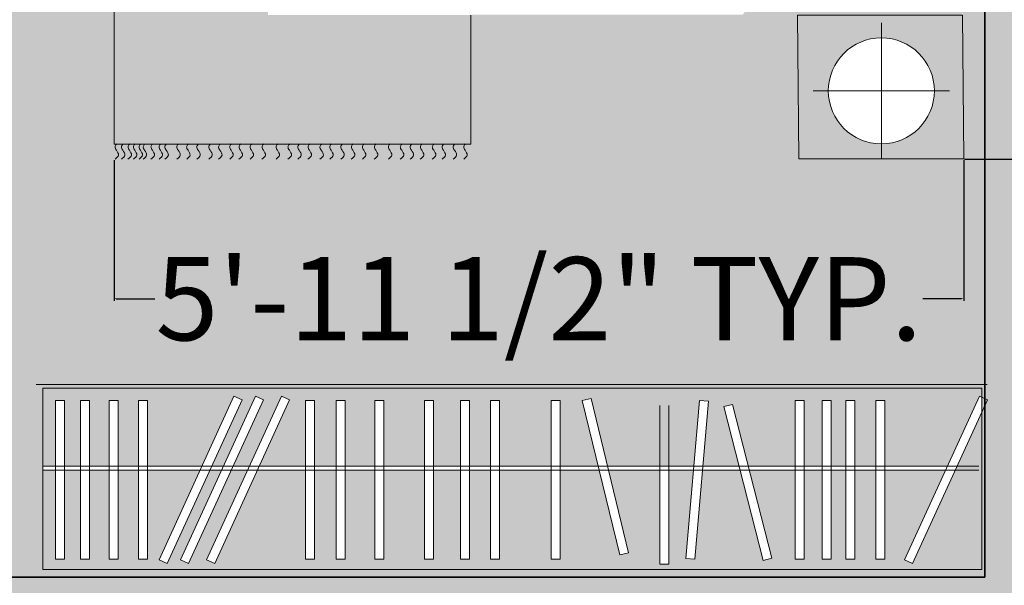
# Model space of a CAD drawing. Units: inches. Extents: x 1316 to 1777, y 813 to 1650.
# Tile 19 of 22: x 1623 to 1706, y 1434 to 1481. Entities that reach past the tile are written whole.
import ezdxf

# ---------------------------------------------------------------- set-up
doc = ezdxf.new("R2010")
doc.units = ezdxf.units.IN
doc.header["$MEASUREMENT"] = 0
for name, color, linetype, lineweight in [('A-ANNO-DIMS', 2, 'Continuous', 18), ('A-FLOR-CASE-PATT', 252, 'Continuous', 13), ('A-FURN-PATT', 23, 'Continuous', 13), ('A-WALL-PATT', 250, 'Continuous', 13), ('closet', 23, 'Continuous', 18), ('furniture', 23, 'Continuous', 18), ('walls', 250, 'Continuous', 35)]:
    doc.layers.add(name, color=color, linetype=linetype, lineweight=lineweight)
doc.layers.add('A-FLOR-PATT', color=254, linetype='Continuous', lineweight=13, true_color=0xfeeab9)
doc.styles.get("Standard").update_dxf_attribs({"font": 'arial.ttf'})
doc.dimstyles.get("Standard").update_dxf_attribs({"dimtxt": 7, "dimasz": 0.18, "dimexe": 0.18, "dimexo": 0.0625, "dimgap": 0.09, "dimtad": 0, "dimtih": 1, "dimtoh": 1, "dimzin": 0, "dimdsep": 46, "dimlunit": 3, "dimtxsty": 'Standard', "dimcen": 0.09, "dimadec": 0, "dimazin": 0, "dimtfac": 1, "dimtofl": 0, "dimtmove": 0, "dimatfit": 3, "dimfxl": 1, "dimtolj": 1, "dimtzin": 0, "dimarcsym": 0})

# ---------------------------------------------------------------- blocks, each defined once
blk = doc.blocks.new('CARPET')
at = {"layer": 'furniture'}
for p, q in [((36, -55.12), (51.55, -55.12)), ((51.55, -55.12), (51.55, -98.11)), ((51.55, -98.11), (-51.53, -98.11))]:
    blk.add_line(p, q, dxfattribs=at)
for points, knots in [([(53.37, -55.99), (53.22, -55.8), (52.9, -55.41), (52.34, -55.8), (51.89, -56.08), (51.65, -55.91), (51.53, -55.83)], [0, 0, 0, 0, 0.653278, 1.290138, 1.740457, 2.114451, 2.114451, 2.114451, 2.114451]), ([(53.37, -57.26), (53.22, -57.07), (52.9, -56.67), (52.34, -57.07), (51.89, -57.35), (51.65, -57.17), (51.53, -57.1)], [0, 0, 0, 0, 0.653278, 1.290138, 1.740457, 2.114451, 2.114451, 2.114451, 2.114451]), ([(53.37, -58.59), (53.22, -58.4), (52.9, -58.01), (52.34, -58.4), (51.89, -58.68), (51.65, -58.5), (51.53, -58.43)], [0, 0, 0, 0, 0.653278, 1.290138, 1.740457, 2.114451, 2.114451, 2.114451, 2.114451]), ([(53.37, -59.78), (53.22, -59.58), (52.9, -59.19), (52.34, -59.58), (51.89, -59.86), (51.65, -59.69), (51.53, -59.61)], [0, 0, 0, 0, 0.653278, 1.290138, 1.740457, 2.114451, 2.114451, 2.114451, 2.114451]), ([(53.37, -61.22), (53.22, -61.02), (52.9, -60.63), (52.34, -61.02), (51.89, -61.3), (51.65, -61.13), (51.53, -61.05)], [0, 0, 0, 0, 0.653278, 1.290138, 1.740457, 2.114451, 2.114451, 2.114451, 2.114451]), ([(53.37, -62.44), (53.22, -62.25), (52.9, -61.86), (52.34, -62.25), (51.89, -62.53), (51.65, -62.36), (51.53, -62.28)], [0, 0, 0, 0, 0.653278, 1.290138, 1.740457, 2.114451, 2.114451, 2.114451, 2.114451]), ([(53.37, -63.63), (53.22, -63.43), (52.9, -63.04), (52.34, -63.43), (51.89, -63.72), (51.65, -63.54), (51.53, -63.46)], [0, 0, 0, 0, 0.653278, 1.290138, 1.740457, 2.114451, 2.114451, 2.114451, 2.114451]), ([(53.37, -65.07), (53.22, -64.87), (52.9, -64.48), (52.34, -64.87), (51.89, -65.15), (51.65, -64.98), (51.53, -64.9)], [0, 0, 0, 0, 0.653278, 1.290138, 1.740457, 2.114451, 2.114451, 2.114451, 2.114451]), ([(53.37, -66.76), (53.22, -66.56), (52.9, -66.17), (52.34, -66.56), (51.89, -66.84), (51.65, -66.67), (51.53, -66.59)], [0, 0, 0, 0, 0.653278, 1.290138, 1.740457, 2.114451, 2.114451, 2.114451, 2.114451]), ([(53.37, -68.2), (53.22, -68), (52.9, -67.61), (52.34, -68), (51.89, -68.28), (51.65, -68.11), (51.53, -68.03)], [0, 0, 0, 0, 0.653278, 1.290138, 1.740457, 2.114451, 2.114451, 2.114451, 2.114451]), ([(53.37, -69.53), (53.22, -69.33), (52.9, -68.94), (52.34, -69.33), (51.89, -69.61), (51.65, -69.44), (51.53, -69.36)], [0, 0, 0, 0, 0.653278, 1.290138, 1.740457, 2.114451, 2.114451, 2.114451, 2.114451]), ([(53.37, -70.79), (53.22, -70.6), (52.9, -70.21), (52.34, -70.6), (51.89, -70.88), (51.65, -70.7), (51.53, -70.63)], [0, 0, 0, 0, 0.653278, 1.290138, 1.740457, 2.114451, 2.114451, 2.114451, 2.114451]), ([(53.37, -72.12), (53.22, -71.93), (52.9, -71.54), (52.34, -71.93), (51.89, -72.21), (51.65, -72.04), (51.53, -71.96)], [0, 0, 0, 0, 0.653278, 1.290138, 1.740457, 2.114451, 2.114451, 2.114451, 2.114451]), ([(53.37, -73.31), (53.22, -73.11), (52.9, -72.72), (52.34, -73.11), (51.89, -73.4), (51.65, -73.22), (51.53, -73.14)], [0, 0, 0, 0, 0.653278, 1.290138, 1.740457, 2.114451, 2.114451, 2.114451, 2.114451]), ([(53.37, -74.75), (53.22, -74.55), (52.9, -74.16), (52.34, -74.55), (51.89, -74.83), (51.65, -74.66), (51.53, -74.58)], [0, 0, 0, 0, 0.653278, 1.290138, 1.740457, 2.114451, 2.114451, 2.114451, 2.114451]), ([(53.37, -75.98), (53.22, -75.78), (52.9, -75.39), (52.34, -75.78), (51.89, -76.06), (51.65, -75.89), (51.53, -75.81)], [0, 0, 0, 0, 0.653278, 1.290138, 1.740457, 2.114451, 2.114451, 2.114451, 2.114451]), ([(53.37, -77.16), (53.22, -76.96), (52.9, -76.57), (52.34, -76.96), (51.89, -77.25), (51.65, -77.07), (51.53, -76.99)], [0, 0, 0, 0, 0.653278, 1.290138, 1.740457, 2.114451, 2.114451, 2.114451, 2.114451]), ([(53.37, -78.6), (53.22, -78.4), (52.9, -78.01), (52.34, -78.4), (51.89, -78.68), (51.65, -78.51), (51.53, -78.43)], [0, 0, 0, 0, 0.653278, 1.290138, 1.740457, 2.114451, 2.114451, 2.114451, 2.114451]), ([(53.37, -80.29), (53.22, -80.09), (52.9, -79.7), (52.34, -80.09), (51.89, -80.37), (51.65, -80.2), (51.53, -80.12)], [0, 0, 0, 0, 0.653278, 1.290138, 1.740457, 2.114451, 2.114451, 2.114451, 2.114451]), ([(53.37, -81.73), (53.22, -81.53), (52.9, -81.14), (52.34, -81.53), (51.89, -81.81), (51.65, -81.64), (51.53, -81.56)], [0, 0, 0, 0, 0.653278, 1.290138, 1.740457, 2.114451, 2.114451, 2.114451, 2.114451]), ([(53.37, -83.06), (53.22, -82.86), (52.9, -82.47), (52.34, -82.86), (51.89, -83.14), (51.65, -82.97), (51.53, -82.89)], [0, 0, 0, 0, 0.653278, 1.290138, 1.740457, 2.114451, 2.114451, 2.114451, 2.114451]), ([(53.37, -84.18), (53.22, -83.99), (52.9, -83.6), (52.34, -83.99), (51.89, -84.27), (51.65, -84.09), (51.53, -84.02)], [0, 0, 0, 0, 0.653278, 1.290138, 1.740457, 2.114451, 2.114451, 2.114451, 2.114451]), ([(53.37, -85.51), (53.22, -85.32), (52.9, -84.93), (52.34, -85.32), (51.89, -85.6), (51.65, -85.42), (51.53, -85.35)], [0, 0, 0, 0, 0.653278, 1.290138, 1.740457, 2.114451, 2.114451, 2.114451, 2.114451]), ([(53.37, -86.7), (53.22, -86.5), (52.9, -86.11), (52.34, -86.5), (51.89, -86.78), (51.65, -86.61), (51.53, -86.53)], [0, 0, 0, 0, 0.653278, 1.290138, 1.740457, 2.114451, 2.114451, 2.114451, 2.114451]), ([(53.37, -88.14), (53.22, -87.94), (52.9, -87.55), (52.34, -87.94), (51.89, -88.22), (51.65, -88.05), (51.53, -87.97)], [0, 0, 0, 0, 0.653278, 1.290138, 1.740457, 2.114451, 2.114451, 2.114451, 2.114451]), ([(53.37, -89.36), (53.22, -89.17), (52.9, -88.78), (52.34, -89.17), (51.89, -89.45), (51.65, -89.28), (51.53, -89.2)], [0, 0, 0, 0, 0.653278, 1.290138, 1.740457, 2.114451, 2.114451, 2.114451, 2.114451]), ([(53.37, -90.55), (53.22, -90.35), (52.9, -89.96), (52.34, -90.35), (51.9, -90.63), (51.66, -90.47), (51.55, -90.4)], [0, 0, 0, 0, 0.653278, 1.290138, 1.740457, 2.0926, 2.0926, 2.0926, 2.0926]), ([(53.37, -91.99), (53.22, -91.79), (52.9, -91.4), (52.34, -91.79), (51.9, -92.07), (51.66, -91.91), (51.55, -91.83)], [0, 0, 0, 0, 0.653278, 1.290138, 1.740457, 2.0926, 2.0926, 2.0926, 2.0926]), ([(53.37, -92.69), (53.22, -92.49), (52.9, -92.09), (52.34, -92.49), (51.9, -92.77), (51.66, -92.61), (51.55, -92.53)], [0, 0, 0, 0, 0.656792, 1.295826, 1.746145, 2.098292, 2.098292, 2.098292, 2.098292]), ([(53.37, -93.66), (53.22, -93.46), (52.9, -93.07), (52.34, -93.46), (51.9, -93.74), (51.66, -93.58), (51.55, -93.5)], [0, 0, 0, 0, 0.653278, 1.290138, 1.740457, 2.0926, 2.0926, 2.0926, 2.0926]), ([(53.37, -94.59), (53.22, -94.4), (52.9, -94.01), (52.34, -94.4), (51.9, -94.68), (51.66, -94.51), (51.55, -94.44)], [0, 0, 0, 0, 0.653278, 1.290138, 1.740457, 2.0926, 2.0926, 2.0926, 2.0926]), ([(53.37, -95.1), (53.22, -94.9), (52.9, -94.51), (52.34, -94.9), (51.9, -95.18), (51.66, -95.02), (51.55, -94.94)], [0, 0, 0, 0, 0.653278, 1.290138, 1.740457, 2.0926, 2.0926, 2.0926, 2.0926]), ([(53.37, -95.78), (53.22, -95.58), (52.9, -95.19), (52.34, -95.58), (51.89, -95.86), (51.65, -95.69), (51.53, -95.61)], [0, 0, 0, 0, 0.653278, 1.290138, 1.740457, 2.114451, 2.114451, 2.114451, 2.114451]), ([(53.37, -96.43), (53.22, -96.23), (52.9, -95.84), (52.34, -96.23), (51.89, -96.51), (51.65, -96.34), (51.53, -96.26)], [0, 0, 0, 0, 0.653278, 1.290138, 1.740457, 2.114451, 2.114451, 2.114451, 2.114451]), ([(53.37, -97.22), (53.22, -97.02), (52.9, -96.63), (52.34, -97.02), (51.89, -97.3), (51.65, -97.13), (51.53, -97.05)], [0, 0, 0, 0, 0.653278, 1.290138, 1.740457, 2.114451, 2.114451, 2.114451, 2.114451]), ([(53.37, -97.99), (53.22, -97.79), (52.9, -97.4), (52.34, -97.79), (51.89, -98.08), (51.65, -97.9), (51.53, -97.82)], [0, 0, 0, 0, 0.653278, 1.290138, 1.740457, 2.114451, 2.114451, 2.114451, 2.114451])]:
    blk.add_open_spline(points, degree=3, knots=knots, dxfattribs=at)
blk = doc.blocks.new('A$C58D270C6')
at = {"layer": 'furniture'}
for p, q in [((9.09, 124.13), (9.09, 108.87)), ((1.46, 116.5), (16.73, 116.5))]:
    blk.add_line(p, q, dxfattribs=at)
blk.add_lwpolyline([(18.5, 108), (18.34, 124.13), (-0.16, 124.13), (0, 108)], close=True, dxfattribs=at)
blk.add_circle((9.09, 116.5), 5.95, dxfattribs=at)
at = {"layer": 'furniture', "xscale": 0.9312884925094044, "yscale": 0.9312884925094044, "zscale": 0.9312884925094044, "rotation": 90}
blk.add_blockref('CARPET', (3.79, 74.47), dxfattribs=at)
blk = doc.blocks.new('closet')
at = {"layer": 'closet'}
for p, q in [((-0.712, -5.577), (5.592, 8.191)), ((6.268, 7.882), (-0.036, -5.886)), ((5.592, 8.191), (6.268, 7.882)), ((7.922, 7.842), (8.679, 7.842)), ((7.922, 7.842), (7.922, -5.515)), ((8.679, 7.842), (8.679, -5.515)), ((10.443, 7.842), (11.2, 7.842)), ((10.443, 7.842), (10.443, -5.515)), ((11.2, 7.842), (11.2, -5.515)), ((12.449, 7.842), (13.206, 7.842)), ((12.449, 7.842), (12.449, -5.515)), ((13.206, 7.842), (13.206, -5.515)), ((14.712, 7.842), (15.469, 7.842)), ((14.712, 7.842), (14.712, -5.515)), ((15.469, 7.842), (15.469, -5.515)), ((17.436, 7.748), (18.17, 7.935)), ((17.436, 7.748), (20.729, -5.196)), ((18.17, 7.935), (21.462, -5.009)), ((23.918, 7.842), (22.755, -5.464)), ((24.672, 7.776), (23.509, -5.53)), ((23.918, 7.842), (24.672, 7.776)), ((26.086, 8.254), (26.086, -5.103)), ((26.843, 8.254), (26.843, -5.103)), ((30.221, 7.465), (33.372, -5.515)), ((35.229, 7.842), (35.229, -5.515)), ((35.986, 7.842), (35.986, -5.515)), ((40.326, 7.842), (40.326, -5.515)), ((41.083, 7.842), (41.083, -5.515)), ((42.848, 7.842), (42.848, -5.515)), ((43.605, 7.842), (43.605, -5.515)), ((45.896, 7.842), (45.896, -5.515)), ((46.653, 7.842), (46.653, -5.515)), ((50.066, 7.842), (50.066, -5.515)), ((50.823, 7.842), (50.823, -5.515)), ((53.325, 7.842), (53.325, -5.515)), ((54.081, 7.842), (54.081, -5.515)), ((55.896, 7.842), (55.896, -5.515)), ((56.653, 7.842), (56.653, -5.515)), ((57.994, -5.577), (64.297, 8.191)), ((64.973, 7.882), (58.669, -5.886)), ((60.189, -5.577), (66.493, 8.191)), ((67.169, 7.882), (60.865, -5.886)), ((61.999, -5.577), (68.303, 8.191)), ((68.978, 7.882), (62.675, -5.886)), ((69.963, 7.842), (69.963, -5.515)), ((70.72, 7.842), (70.72, -5.515)), ((72.429, 7.842), (72.429, -5.515)), ((73.186, 7.842), (73.186, -5.515)), ((74.817, 7.842), (74.817, -5.515)), ((75.574, 7.842), (75.574, -5.515)), ((76.936, 7.842), (76.936, -5.515)), ((77.693, 7.842), (77.693, -5.515)), ((-0.232, 7.394), (-0.232, -6.566)), ((29.485, 7.286), (32.636, -5.694)), ((56.234, 0.335), (0, 0.335)), ((56.2, 0), (0, 0)), ((56.2, 0), (78.757, 0)), ((56.234, 0.335), (78.757, 0.335)), ((-0.036, -5.886), (-0.712, -5.577)), ((21.462, -5.009), (20.729, -5.196)), ((23.509, -5.53), (22.755, -5.464)), ((33.372, -5.515), (32.636, -5.694)), ((35.986, -5.515), (35.229, -5.515)), ((41.083, -5.515), (40.326, -5.515)), ((43.605, -5.515), (42.848, -5.515)), ((46.653, -5.515), (45.896, -5.515)), ((50.823, -5.515), (50.066, -5.515)), ((54.081, -5.515), (53.325, -5.515)), ((56.653, -5.515), (55.896, -5.515)), ((58.669, -5.886), (57.994, -5.577)), ((60.865, -5.886), (60.189, -5.577)), ((62.675, -5.886), (61.999, -5.577)), ((70.72, -5.515), (69.963, -5.515)), ((73.186, -5.515), (72.429, -5.515)), ((75.574, -5.515), (74.817, -5.515)), ((77.693, -5.515), (76.936, -5.515))]:
    blk.add_line(p, q, dxfattribs=at)
blk = doc.blocks.new('rotated closet')
at = {"layer": 'closet'}
for p, q in [((26.318, 0.86), (27.074, 0.86)), ((29.717, -0.108), (30.452, 0.071)), ((35.461, 0.448), (36.217, 0.448)), ((40.558, 0.448), (41.314, 0.448)), ((43.08, 0.448), (43.837, 0.448)), ((46.128, 0.448), (46.884, 0.448)), ((50.298, 0.448), (51.055, 0.448)), ((53.556, 0.448), (54.313, 0.448)), ((56.128, 0.448), (56.884, 0.448)), ((64.529, 0.797), (65.205, 0.488)), ((66.725, 0.797), (67.4, 0.488)), ((68.534, 0.797), (69.21, 0.488)), ((70.195, 0.448), (70.952, 0.448)), ((72.66, 0.448), (73.417, 0.448)), ((75.049, 0.448), (75.806, 0.448)), ((77.168, 0.448), (77.924, 0.448)), ((78.989, 0), (78.989, -13.96)), ((8.91, -12.909), (8.153, -12.909)), ((11.431, -12.909), (10.675, -12.909)), ((13.437, -12.909), (12.681, -12.909)), ((15.7, -12.909), (14.943, -12.909)), ((0, -13.96), (78.989, -13.96)), ((-0.456, -14.274), (79.544, -14.274))]:
    blk.add_line(p, q, dxfattribs=at)
blk.add_blockref('closet', (0.232, -7.394), dxfattribs=at)
blk = doc.blocks.new('WARDROBE-80')
for p, q in [((80, 15.567), (0, 15.567)), ((80, 15.567), (0, 15.567)), ((80, 15.567), (0, 15.567)), ((0.555, 15.252), (0.555, 0.442)), ((79.544, 15.252), (0.555, 15.252)), ((79.544, 15.252), (2.199, 15.252)), ((79.544, 0), (79.544, 15.252)), ((0.555, 0), (0.555, 0.442)), ((79.544, 0), (0.555, 0))]:
    blk.add_line(p, q)
at = {"rotation": 179.9999999959433}
blk.add_blockref('rotated closet', (79.544, 1.293), dxfattribs=at)
blk = doc.blocks.new('*D28')
at = {"layer": 'A-ANNO-DIMS', "color": 0, "lineweight": -2, "transparency": 16777216}
for p, q in [((1702.469, 1547.775), (1714.322, 1547.775)), ((1714.142, 1547.595), (1714.142, 1512.322)), ((1714.142, 1469.722), (1714.142, 1504.994)), ((1702.469, 1469.542), (1714.322, 1469.542))]:
    blk.add_line(p, q, dxfattribs=at)
at = {"layer": 'A-ANNO-DIMS', "color": 0, "transparency": 16777216}
for points in [[(1714.112, 1547.595), (1714.172, 1547.595), (1714.142, 1547.775)], [(1714.112, 1469.722), (1714.172, 1469.722), (1714.142, 1469.542)]]:
    blk.add_solid(points, dxfattribs=at)
at = {"layer": 'Defpoints', "color": 0, "transparency": 16777216}
for p in [(1702.407, 1547.775), (1702.407, 1469.542), (1714.142, 1469.542)]:
    blk.add_point(p, dxfattribs=at)
at = {"layer": 'A-ANNO-DIMS', "color": 0, "transparency": 16777216, "insert": (1714.142, 1508.658), "char_height": 7, "attachment_point": 5}
blk.add_mtext('\\A1;BED 6\'-6" TYP.', dxfattribs=at)
blk = doc.blocks.new('*D29')
at = {"layer": 'A-ANNO-DIMS', "color": 0, "lineweight": -2, "transparency": 16777216}
for p, q in [((1630.921, 1469.479), (1630.921, 1457.627)), ((1702.407, 1469.479), (1702.407, 1457.627)), ((1631.101, 1457.807), (1634.365, 1457.807)), ((1702.227, 1457.807), (1698.963, 1457.807))]:
    blk.add_line(p, q, dxfattribs=at)
at = {"layer": 'A-ANNO-DIMS', "color": 0, "transparency": 16777216}
for points in [[(1631.101, 1457.837), (1631.101, 1457.777), (1630.921, 1457.807)], [(1702.227, 1457.837), (1702.227, 1457.777), (1702.407, 1457.807)]]:
    blk.add_solid(points, dxfattribs=at)
at = {"layer": 'Defpoints', "color": 0, "transparency": 16777216}
for p in [(1630.921, 1469.542), (1702.407, 1469.542), (1630.921, 1457.807)]:
    blk.add_point(p, dxfattribs=at)
at = {"layer": 'A-ANNO-DIMS', "color": 0, "transparency": 16777216, "insert": (1666.664, 1457.807), "char_height": 7, "attachment_point": 5}
blk.add_mtext('\\A1;5\'-11 1/2" TYP.', dxfattribs=at)

msp = doc.modelspace()

# ---------------------------------------------------------------- hatches: boundary and pattern name
at = {"layer": 'A-FLOR-CASE-PATT'}
h = msp.add_hatch(color=256, dxfattribs=at)
h.dxf.hatch_style = 1
h.paths.add_polyline_path([(1641.013, 1449.6), (1641.689, 1449.29), (1639.136, 1443.714), (1640.128, 1443.714), (1642.823, 1449.6), (1643.499, 1449.29), (1640.945, 1443.714), (1642.323, 1443.714), (1645.018, 1449.6), (1645.694, 1449.29), (1643.141, 1443.714), (1647.035, 1443.714), (1647.035, 1449.229), (1647.792, 1449.229), (1647.792, 1443.714), (1649.606, 1443.714), (1649.606, 1449.229), (1650.363, 1449.229), (1650.363, 1443.714), (1652.865, 1443.714), (1652.865, 1449.229), (1653.621, 1449.229), (1653.621, 1443.714), (1657.035, 1443.714), (1657.035, 1449.229), (1657.792, 1449.229), (1657.792, 1443.714), (1660.083, 1443.714), (1660.083, 1449.229), (1660.839, 1449.229), (1660.839, 1443.714), (1662.605, 1443.714), (1662.605, 1449.229), (1663.362, 1449.229), (1663.362, 1443.714), (1667.702, 1443.714), (1667.702, 1449.229), (1668.459, 1449.229), (1668.459, 1443.714), (1671.655, 1443.714), (1670.316, 1449.229), (1671.051, 1449.407), (1672.434, 1443.714), (1679.696, 1443.714), (1680.179, 1449.244), (1680.933, 1449.178), (1680.455, 1443.714), (1683.5, 1443.714), (1682.225, 1448.723), (1682.959, 1448.91), (1684.281, 1443.714), (1688.219, 1443.714), (1688.219, 1449.229), (1688.976, 1449.229), (1688.976, 1443.714), (1690.482, 1443.714), (1690.482, 1449.229), (1691.239, 1449.229), (1691.239, 1443.714), (1692.488, 1443.714), (1692.488, 1449.229), (1693.245, 1449.229), (1693.245, 1443.714), (1695.009, 1443.714), (1695.009, 1449.229), (1695.766, 1449.229), (1695.766, 1443.714), (1701.029, 1443.714), (1703.724, 1449.6), (1703.919, 1449.51), (1703.919, 1450.279), (1624.931, 1450.279), (1624.931, 1443.714), (1625.995, 1443.714), (1625.995, 1449.229), (1626.752, 1449.229), (1626.752, 1443.714), (1628.114, 1443.714), (1628.114, 1449.229), (1628.871, 1449.229), (1628.871, 1443.714), (1630.502, 1443.714), (1630.502, 1449.229), (1631.259, 1449.229), (1631.259, 1443.714), (1632.968, 1443.714), (1632.968, 1449.229), (1633.724, 1449.229), (1633.724, 1443.714), (1638.318, 1443.714)])
h.paths.add_polyline_path([(1638.165, 1443.379), (1633.724, 1443.379), (1633.724, 1435.872), (1632.968, 1435.872), (1632.968, 1443.379), (1631.259, 1443.379), (1631.259, 1435.872), (1630.502, 1435.872), (1630.502, 1443.379), (1628.871, 1443.379), (1628.871, 1435.872), (1628.114, 1435.872), (1628.114, 1443.379), (1626.752, 1443.379), (1626.752, 1435.872), (1625.995, 1435.872), (1625.995, 1443.379), (1624.931, 1443.379), (1624.931, 1436.32), (1624.931, 1435.469), (1624.931, 1435.026), (1703.919, 1435.026), (1703.919, 1448.241), (1698.096, 1435.522), (1697.42, 1435.832), (1700.875, 1443.379), (1695.766, 1443.379), (1695.766, 1435.872), (1695.009, 1435.872), (1695.009, 1443.379), (1693.245, 1443.379), (1693.245, 1435.872), (1692.488, 1435.872), (1692.488, 1443.379), (1691.239, 1443.379), (1691.239, 1435.872), (1690.482, 1435.872), (1690.482, 1443.379), (1688.976, 1443.379), (1688.976, 1435.872), (1688.219, 1435.872), (1688.219, 1443.379), (1684.366, 1443.379), (1686.252, 1435.965), (1685.518, 1435.779), (1683.585, 1443.379), (1680.426, 1443.379), (1679.77, 1435.872), (1679.016, 1435.938), (1679.666, 1443.379), (1677.602, 1443.379), (1677.602, 1435.46), (1676.845, 1435.46), (1676.845, 1443.379), (1672.515, 1443.379), (1674.202, 1436.427), (1673.467, 1436.249), (1671.736, 1443.379), (1668.459, 1443.379), (1668.459, 1435.872), (1667.702, 1435.872), (1667.702, 1443.379), (1663.362, 1443.379), (1663.362, 1435.872), (1662.605, 1435.872), (1662.605, 1443.379), (1660.839, 1443.379), (1660.839, 1435.872), (1660.083, 1435.872), (1660.083, 1443.379), (1657.792, 1443.379), (1657.792, 1435.872), (1657.035, 1435.872), (1657.035, 1443.379), (1653.621, 1443.379), (1653.621, 1435.872), (1652.865, 1435.872), (1652.865, 1443.379), (1650.363, 1443.379), (1650.363, 1435.872), (1649.606, 1435.872), (1649.606, 1443.379), (1647.792, 1443.379), (1647.792, 1435.872), (1647.035, 1435.872), (1647.035, 1443.379), (1642.988, 1443.379), (1639.39, 1435.522), (1638.715, 1435.832), (1642.17, 1443.379), (1640.792, 1443.379), (1637.195, 1435.522), (1636.519, 1435.832), (1639.974, 1443.379), (1638.983, 1443.379), (1635.385, 1435.522), (1634.709, 1435.832)])
at = {"layer": 'A-FLOR-PATT'}
h = msp.add_hatch(color=256, dxfattribs=at)
h.dxf.hatch_style = 1
h.paths.add_polyline_path([(1704.173, 1566.369), (1574.845, 1566.369), (1574.845, 1434.369), (1704.173, 1434.369)])
h.paths.add_polyline_path([(1630.932, 1542.856), (1660.956, 1542.856), (1660.956, 1535.716), (1688.427, 1535.716), (1688.322, 1546.604), (1686.085, 1547.859), (1686.091, 1547.88), (1685.166, 1550.963), (1681.619, 1555.397), (1678.246, 1552.474), (1678.253, 1552.433), (1678.187, 1552.423), (1681.619, 1555.397), (1683.601, 1556.058), (1683.639, 1556.172), (1683.764, 1556.112), (1686.94, 1557.171), (1688.039, 1558.585), (1688.034, 1558.699), (1688.108, 1558.672), (1686.969, 1557.208), (1686.965, 1557.18), (1681.619, 1555.397), (1682.039, 1554.872), (1682.12, 1554.846), (1682.107, 1554.788), (1685.145, 1550.989), (1685.188, 1550.977), (1685.173, 1550.941), (1685.764, 1548.971), (1688.364, 1547.814), (1702.185, 1547.814), (1702.301, 1535.716), (1702.301, 1481.716), (1702.418, 1469.617), (1688.544, 1469.617), (1688.427, 1481.716), (1660.956, 1481.716), (1660.956, 1470.853), (1630.932, 1470.853)], flags=16)
h.paths.add_polyline_path([(1624.931, 1450.279), (1703.919, 1450.279), (1703.919, 1436.32), (1703.919, 1435.026), (1624.931, 1435.026), (1624.931, 1435.469)], flags=16)
h.paths.add_polyline_path([(1624.931, 1443.714), (1625.995, 1443.714), (1625.995, 1449.229), (1626.752, 1449.229), (1626.752, 1443.714), (1628.114, 1443.714), (1628.114, 1449.229), (1628.871, 1449.229), (1628.871, 1443.714), (1630.502, 1443.714), (1630.502, 1449.229), (1631.259, 1449.229), (1631.259, 1443.714), (1632.968, 1443.714), (1632.968, 1449.229), (1633.724, 1449.229), (1633.724, 1443.714), (1638.318, 1443.714), (1641.013, 1449.6), (1641.689, 1449.29), (1639.136, 1443.714), (1640.128, 1443.714), (1642.823, 1449.6), (1643.499, 1449.29), (1640.945, 1443.714), (1642.323, 1443.714), (1645.018, 1449.6), (1645.694, 1449.29), (1643.141, 1443.714), (1647.035, 1443.714), (1647.035, 1449.229), (1647.792, 1449.229), (1647.792, 1443.714), (1649.606, 1443.714), (1649.606, 1449.229), (1650.363, 1449.229), (1650.363, 1443.714), (1652.865, 1443.714), (1652.865, 1449.229), (1653.621, 1449.229), (1653.621, 1443.714), (1657.035, 1443.714), (1657.035, 1449.229), (1657.792, 1449.229), (1657.792, 1443.714), (1660.083, 1443.714), (1660.083, 1449.229), (1660.839, 1449.229), (1660.839, 1443.714), (1662.605, 1443.714), (1662.605, 1449.229), (1663.362, 1449.229), (1663.362, 1443.714), (1667.702, 1443.714), (1667.702, 1449.229), (1668.459, 1449.229), (1668.459, 1443.714), (1671.655, 1443.714), (1670.316, 1449.229), (1671.051, 1449.407), (1672.434, 1443.714), (1679.696, 1443.714), (1680.179, 1449.244), (1680.933, 1449.178), (1680.455, 1443.714), (1683.5, 1443.714), (1682.225, 1448.723), (1682.959, 1448.91), (1684.281, 1443.714), (1688.219, 1443.714), (1688.219, 1449.229), (1688.976, 1449.229), (1688.976, 1443.714), (1690.482, 1443.714), (1690.482, 1449.229), (1691.239, 1449.229), (1691.239, 1443.714), (1692.488, 1443.714), (1692.488, 1449.229), (1693.245, 1449.229), (1693.245, 1443.714), (1695.009, 1443.714), (1695.009, 1449.229), (1695.766, 1449.229), (1695.766, 1443.714), (1701.029, 1443.714), (1700.875, 1443.379), (1695.766, 1443.379), (1695.766, 1435.872), (1695.009, 1435.872), (1695.009, 1443.379), (1693.245, 1443.379), (1693.245, 1435.872), (1692.488, 1435.872), (1692.488, 1443.379), (1691.239, 1443.379), (1691.239, 1435.872), (1690.482, 1435.872), (1690.482, 1443.379), (1688.976, 1443.379), (1688.976, 1435.872), (1688.219, 1435.872), (1688.219, 1443.379), (1684.366, 1443.379), (1686.252, 1435.965), (1685.518, 1435.779), (1683.585, 1443.379), (1680.426, 1443.379), (1679.77, 1435.872), (1679.016, 1435.938), (1679.666, 1443.379), (1677.602, 1443.379), (1677.602, 1435.46), (1676.845, 1435.46), (1676.845, 1443.379), (1672.515, 1443.379), (1674.202, 1436.427), (1673.467, 1436.249), (1671.736, 1443.379), (1668.459, 1443.379), (1668.459, 1435.872), (1667.702, 1435.872), (1667.702, 1443.379), (1663.362, 1443.379), (1663.362, 1435.872), (1662.605, 1435.872), (1662.605, 1443.379), (1660.839, 1443.379), (1660.839, 1435.872), (1660.083, 1435.872), (1660.083, 1443.379), (1657.792, 1443.379), (1657.792, 1435.872), (1657.035, 1435.872), (1657.035, 1443.379), (1653.621, 1443.379), (1653.621, 1435.872), (1652.865, 1435.872), (1652.865, 1443.379), (1650.363, 1443.379), (1650.363, 1435.872), (1649.606, 1435.872), (1649.606, 1443.379), (1647.792, 1443.379), (1647.792, 1435.872), (1647.035, 1435.872), (1647.035, 1443.379), (1642.988, 1443.379), (1639.39, 1435.522), (1638.715, 1435.832), (1642.17, 1443.379), (1640.792, 1443.379), (1637.195, 1435.522), (1636.519, 1435.832), (1639.974, 1443.379), (1638.983, 1443.379), (1635.385, 1435.522), (1634.709, 1435.832), (1638.165, 1443.379), (1633.724, 1443.379), (1633.724, 1435.872), (1632.968, 1435.872), (1632.968, 1443.379), (1631.259, 1443.379), (1631.259, 1435.872), (1630.502, 1435.872), (1630.502, 1443.379), (1628.871, 1443.379), (1628.871, 1435.872), (1628.114, 1435.872), (1628.114, 1443.379), (1626.752, 1443.379), (1626.752, 1435.872), (1625.995, 1435.872), (1625.995, 1443.379), (1624.931, 1443.379)], flags=0)
h.paths.add_polyline_path([(1683.839, 1491.517), (1691.022, 1491.517), (1691.071, 1491.582), (1691.071, 1529.618), (1699.231, 1529.618), (1699.231, 1513.795), (1691.071, 1513.795), (1691.071, 1507.34), (1699.231, 1507.34), (1699.231, 1491.517), (1691.022, 1491.517), (1683.839, 1481.774)], flags=0)
h.paths.add_polyline_path([(1691.015, 1475.341, -1), (1699.947, 1475.341, -1)], flags=0)
h.paths.add_polyline_path([(1690.898, 1541.439, -1), (1699.83, 1541.439, -1)], flags=0)
h.paths.add_polyline_path([(1505.845, 1469.591), (1505.845, 1566.369), (1386.064, 1566.369), (1386.064, 1450.329), (1465.697, 1450.329), (1465.697, 1449.245), (1466.177, 1449.025), (1465.697, 1447.977), (1465.697, 1436.055), (1465.697, 1434.369), (1505.845, 1434.369), (1505.845, 1440.551), (1476.949, 1440.551), (1476.949, 1441.822), (1476.977, 1441.822, -0.400014)])
edge = h.paths.add_edge_path(flags=16)
edge.add_spline(control_points=[(1456.973, 1471.794), (1457.023, 1471.721), (1457.138, 1471.554), (1456.942, 1471.242), (1456.67, 1470.851), (1456.943, 1470.632), (1457.081, 1470.522)], knot_values=[0, 0, 0, 0, 0.352144, 0.802463, 1.439322, 2.0926, 2.0926, 2.0926, 2.0926], degree=3, periodic=0)
edge.add_spline(control_points=[(1457.325, 1471.794), (1457.375, 1471.721), (1457.49, 1471.554), (1457.294, 1471.242), (1457.022, 1470.851), (1457.295, 1470.632), (1457.433, 1470.522)], knot_values=[0, 0, 0, 0, 0.352144, 0.802463, 1.439322, 2.0926, 2.0926, 2.0926, 2.0926], degree=3, periodic=0)
edge = h.paths.add_edge_path(flags=16)
edge.add_line((1429.513, 1471.794), (1429.513, 1482.657))
edge.add_line((1429.513, 1482.657), (1402.042, 1482.657))
edge.add_line((1402.042, 1482.657), (1401.925, 1470.559))
edge.add_line((1401.925, 1470.559), (1388.051, 1470.559))
edge.add_line((1388.051, 1470.559), (1388.167, 1482.657))
edge.add_line((1388.167, 1482.657), (1388.167, 1536.657))
edge.add_line((1388.167, 1536.657), (1388.284, 1548.755))
edge.add_line((1388.284, 1548.755), (1402.158, 1548.755))
edge.add_line((1402.158, 1548.755), (1402.042, 1536.657))
edge.add_line((1402.042, 1536.657), (1429.513, 1536.657))
edge.add_line((1429.513, 1536.657), (1429.513, 1543.797))
edge.add_line((1429.513, 1543.797), (1456.932, 1543.797))
edge.add_spline(control_points=[(1456.932, 1543.797), (1456.987, 1543.874), (1457.108, 1544.044), (1456.911, 1544.361), (1456.638, 1544.752), (1456.911, 1544.971), (1457.049, 1545.082)], knot_values=[0, 0, 0, 0, 0.373994, 0.824314, 1.461173, 2.114451, 2.114451, 2.114451, 2.114451], degree=3, periodic=0)
edge.add_spline(control_points=[(1457.401, 1545.082), (1457.263, 1544.971), (1456.99, 1544.752), (1457.263, 1544.361), (1457.46, 1544.044), (1457.339, 1543.874), (1457.284, 1543.797)], knot_values=[0, 0, 0, 0, 0.653278, 1.290138, 1.740457, 2.114451, 2.114451, 2.114451, 2.114451], degree=3, periodic=0)
edge.add_line((1457.284, 1543.797), (1459.536, 1543.797))
edge.add_line((1459.536, 1543.797), (1459.536, 1471.794))
edge.add_line((1459.536, 1471.794), (1429.513, 1471.794))
h.paths.add_polyline_path([(1406.63, 1482.715), (1399.446, 1492.458), (1399.398, 1492.458), (1391.238, 1492.458), (1391.238, 1508.281), (1399.398, 1508.281), (1399.398, 1514.736), (1391.238, 1514.736), (1391.238, 1530.559), (1399.398, 1530.559), (1399.398, 1492.524), (1399.446, 1492.458), (1406.63, 1492.458)], flags=0)
h.paths.add_polyline_path([(1399.454, 1476.282, -1), (1390.522, 1476.282, -1)], flags=0)
h.paths.add_polyline_path([(1390.638, 1542.38, -1), (1399.571, 1542.38, -1)], flags=0)
h.paths.add_polyline_path([(1487.293, 1548.286), (1487.08, 1548.252), (1487.104, 1547.964)], flags=16)
h.paths.add_polyline_path([(1491.493, 1552.843), (1490.887, 1552.654), (1490.949, 1552.372)], flags=16)
h.paths.add_polyline_path([(1489.966, 1554.409), (1489.859, 1554.561), (1489.718, 1554.445)], flags=16)
h.paths.add_polyline_path([(1497.301, 1546.483), (1497.294, 1546.462), (1497.309, 1546.453)], flags=16)
h.paths.add_polyline_path([(1496.386, 1549.553), (1492.828, 1554), (1492.655, 1554.939), (1492.454, 1555.029), (1492.589, 1555.296), (1491.806, 1559.547), (1491.869, 1559.506), (1491.824, 1559.451), (1492.828, 1554), (1494.81, 1554.661), (1494.848, 1554.774), (1494.973, 1554.715), (1496.01, 1555.061), (1496.078, 1555.314), (1496.341, 1555.171), (1498.15, 1555.774), (1499.249, 1557.187), (1499.243, 1557.301), (1499.317, 1557.275), (1498.179, 1555.811), (1498.174, 1555.782), (1492.828, 1554), (1493.249, 1553.474), (1493.33, 1553.449), (1493.316, 1553.39), (1495.203, 1551.032), (1495.702, 1550.957), (1495.574, 1550.568), (1496.354, 1549.592), (1496.397, 1549.58)], flags=16)
h.paths.add_polyline_path([(1486.021, 1555.224), (1485.958, 1555.549), (1483.595, 1557.912), (1483.28, 1557.859), (1483.243, 1558.264), (1486.27, 1555.237)], flags=16)
h.paths.add_polyline_path([(1505.845, 1469.591, 0.400014), (1476.977, 1441.822), (1505.845, 1441.822)], flags=17)
at = {"layer": 'A-FURN-PATT'}
h = msp.add_hatch(color=256, dxfattribs=at)
h.dxf.hatch_style = 1
h.paths.add_polyline_path([(1688.416, 1481.677), (1702.29, 1481.677), (1702.407, 1469.579), (1695.469, 1469.579), (1695.469, 1470.836, 0.414214), (1699.936, 1475.302, 1), (1691.003, 1475.302, 0.414214), (1695.469, 1470.836), (1695.469, 1469.579), (1688.532, 1469.579)])
h.paths.add_polyline_path([(1691.011, 1491.478), (1699.219, 1491.478), (1699.219, 1507.301), (1691.059, 1507.301), (1691.059, 1513.757), (1699.219, 1513.757), (1699.219, 1529.579), (1691.059, 1529.579), (1691.059, 1535.677), (1702.29, 1535.677), (1702.29, 1481.677), (1683.827, 1481.677), (1683.827, 1481.735)])
h.paths.add_polyline_path([(1690.887, 1541.4, 0.414214), (1695.353, 1536.934), (1695.353, 1535.677), (1688.416, 1535.677), (1688.299, 1547.775), (1702.173, 1547.775), (1702.29, 1535.677), (1695.353, 1535.677), (1695.353, 1536.934, 0.414214), (1699.819, 1541.4, 1)])
h = msp.add_hatch(color=256, dxfattribs=at)
h.dxf.hatch_style = 1
h.paths.add_polyline_path([(1691.059, 1507.301), (1699.219, 1507.301), (1699.219, 1491.478), (1691.059, 1491.478)])
h.paths.add_polyline_path([(1691.059, 1529.579), (1699.219, 1529.579), (1699.219, 1513.757), (1691.059, 1513.757)])
h.paths.add_polyline_path([(1630.921, 1542.817), (1660.945, 1542.817), (1660.945, 1535.677), (1643.861, 1535.677), (1643.861, 1481.677), (1660.945, 1481.677), (1660.945, 1470.814), (1630.921, 1470.814)])
at = {"layer": 'A-WALL-PATT'}
h = msp.add_hatch(color=256, dxfattribs=at)
h.dxf.hatch_style = 1
h.paths.add_polyline_path([(1713.173, 1281.369), (1656.173, 1281.369), (1656.173, 1298.258), (1651.673, 1298.258), (1651.673, 1281.369), (1567.673, 1281.369), (1567.673, 1266.995), (1572.173, 1266.995), (1572.173, 1276.869), (1704.173, 1276.869), (1704.173, 1132.869), (1608.64, 1132.869), (1608.64, 1123.869), (1704.173, 1123.869), (1704.173, 1040.173), (1652.869, 1040.173), (1652.869, 1031.173), (1713.173, 1031.173), (1713.173, 1040.173)])
h.paths.add_polyline_path([(1572.173, 1237.955), (1567.673, 1237.955), (1567.673, 1123.869), (1583.146, 1123.869), (1583.146, 1132.869), (1572.173, 1132.869)], flags=17)
h.paths.add_polyline_path([(1510.345, 1566.369), (1524.171, 1566.369), (1524.171, 1571.985), (1524.171, 1575.369), (1445.955, 1575.369), (1445.955, 1566.369), (1505.845, 1566.369), (1505.845, 1469.591), (1510.345, 1469.591), (1510.345, 1471.869), (1529.081, 1471.869), (1529.081, 1476.369), (1510.345, 1476.369)])
h.paths.add_polyline_path([(1609.722, 1575.369), (1545.119, 1575.369), (1545.119, 1566.369), (1570.345, 1566.369), (1570.345, 1476.369), (1562.477, 1476.369), (1562.477, 1471.869), (1570.345, 1471.869), (1570.345, 1469.591), (1574.845, 1469.591), (1574.845, 1566.369), (1609.722, 1566.369)])
h.paths.add_polyline_path([(1713.173, 1575.369), (1655.233, 1575.369), (1655.233, 1566.369), (1704.173, 1566.369), (1704.173, 1434.369), (1574.845, 1434.369), (1574.845, 1440.551), (1574.701, 1440.551), (1570.345, 1440.551), (1570.345, 1429.869), (1597.673, 1429.869), (1597.673, 1408.281), (1602.173, 1408.281), (1602.173, 1429.869), (1704.173, 1429.869), (1704.173, 1410.704), (1707.375, 1410.704), (1713.173, 1410.704)])
h.paths.add_polyline_path([(1713.173, 1383.676), (1704.173, 1383.676), (1704.173, 1369.869), (1602.173, 1369.869), (1602.173, 1379.241), (1597.673, 1379.241), (1597.673, 1365.369), (1713.173, 1365.369)])
h.paths.add_polyline_path([(1444.564, 1429.869), (1510.345, 1429.869), (1510.345, 1440.551), (1505.845, 1440.551), (1505.845, 1434.369), (1386.064, 1434.369), (1386.064, 1566.369), (1400.445, 1566.369), (1400.445, 1575.369), (1377.064, 1575.369), (1377.064, 1412.813), (1380.509, 1412.813), (1386.064, 1412.813), (1386.064, 1429.869), (1440.064, 1429.869), (1440.064, 1401.229), (1444.564, 1401.229)])
h.paths.add_polyline_path([(1444.564, 1372.189), (1440.064, 1372.189), (1440.064, 1369.869), (1386.064, 1369.869), (1386.064, 1378.758), (1377.064, 1378.758), (1377.064, 1349.201), (1381.118, 1349.201), (1386.064, 1349.201), (1386.064, 1365.369), (1440.064, 1365.369), (1440.064, 1322.882), (1444.564, 1322.882)])
h.paths.add_polyline_path([(1510.564, 1295.094), (1506.064, 1295.094), (1506.064, 1245.369), (1386.064, 1245.369), (1386.064, 1272.582), (1377.064, 1272.582), (1377.064, 1212.905), (1380.1, 1212.905), (1386.064, 1212.905), (1386.064, 1240.869), (1510.564, 1240.869)])
h.paths.add_polyline_path([(1386.064, 1163.761), (1377.064, 1163.761), (1377.064, 1063.869), (1419.363, 1063.869), (1419.363, 1072.869), (1386.064, 1072.869)])
h.paths.add_polyline_path([(1510.564, 1072.869), (1469.381, 1072.869), (1469.381, 1063.869), (1501.564, 1063.869), (1501.564, 1033.023), (1501.564, 1031.173), (1540.829, 1031.173), (1540.829, 1036.182, -0.029954), (1541.068, 1040.173), (1510.564, 1040.173)])
h.paths.add_polyline_path([(1607.369, 1040.173), (1574.225, 1040.173), (1574.225, 1036.182), (1574.225, 1031.173), (1607.369, 1031.173)], flags=17)
h.paths.add_polyline_path([(1637.054, 1040.173), (1624.706, 1040.173), (1624.706, 1031.173), (1637.054, 1031.173)], flags=17)

# ---------------------------------------------------------------- linework, layer by layer
at = {"layer": 'walls'}
for p in [(1704.173, 1566.369), (1574.845, 1434.369)]:
    msp.add_line(p, (1704.173, 1434.369), dxfattribs=at)

# ---------------------------------------------------------------- block references
at = {"layer": 'closet'}
msp.add_blockref('WARDROBE-80', (1624.375, 1435.027), dxfattribs=at)
at = {"layer": 'furniture', "xscale": 0.7500000390647866, "yscale": 0.7500000390647866, "zscale": 0.7500000390647866, "rotation": 180}
msp.add_blockref('A$C58D270C6', (1702.29, 1562.677), dxfattribs=at)

# ---------------------------------------------------------------- dimensions: what is measured, and where the dimension line sits
at = {"layer": 'A-ANNO-DIMS'}
for base, p1, p2, angle, text, picture, middle in [((1714.142, 1469.542), (1702.407, 1547.775), (1702.407, 1469.542), 270, 'BED <> TYP.', '*D28', (1714.142, 1508.658)), ((1630.921, 1457.807), (1702.407, 1469.542), (1630.921, 1469.542), 180, '<> TYP.', '*D29', (1666.664, 1457.807))]:
    dim = msp.add_linear_dim(base=base, p1=p1, p2=p2, angle=angle, text=text, dimstyle='Standard', override={"dimdec": 1, "dimlfac": 1, "dimrnd": 0, "dimzin": 1, "dimdsep": 46, "dimlunit": 4, "dimfrac": 2}, dxfattribs=at)
    dim.commit()
    dim.dimension.update_dxf_attribs({"geometry": picture, "text_midpoint": middle})

doc.saveas('drawing.dxf')
